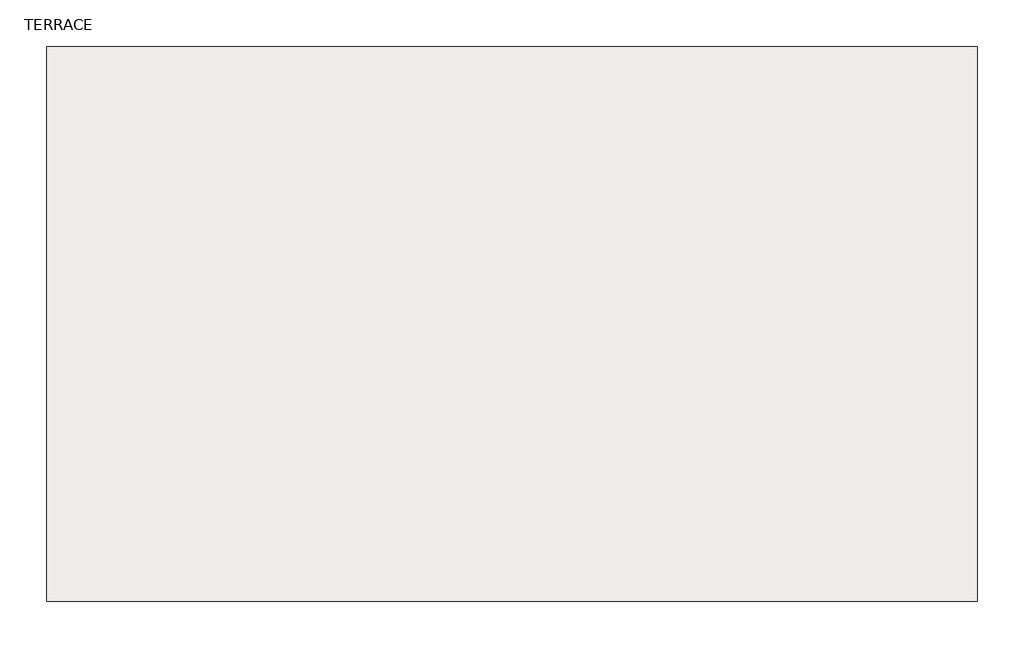
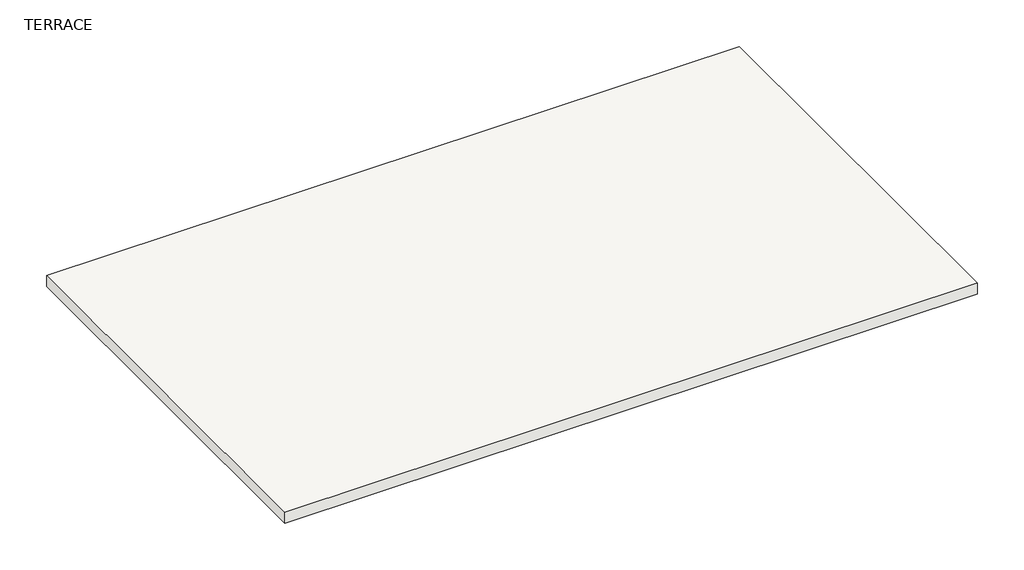
# One storey: 1 slab.
"""IFC4 building model written with IfcOpenShell, lengths in millimetres."""

from ifc_helpers import new_model, si_unit, frame, origin, place, context, project, spatial, polyline, outline, extrude, element, save

model = new_model("IFC4")

# Units and contexts
model_context = context("Model", 3, world=origin())
ifc_project = project(units=[si_unit("LENGTHUNIT", "METRE", prefix="MILLI")], contexts=[model_context])

# Site, building, storey
site = spatial("IfcSite", under=ifc_project)
building = spatial("IfcBuilding", under=site)
storey = spatial("IfcBuildingStorey", under=building, Name="TERRACE", Elevation=12801.6)

# Slab
placement = place(None, origin())
element("IfcSlab", 1, ObjectType="6\" SLAB", at=placement, inside=storey, context=model_context, shape_type="SweptSolid", body=[
    extrude(outline(polyline([(56.4408773, 5407.3642852), (9213.1408773, 5407.3642852), (9213.1408773, -53.6357148), (56.4408773, -53.6357148), (56.4408773, 5407.3642852)])), frame((0.0, 0.0, 12700.0), z_axis=(0.0, 0.0, 1.0), x_axis=(1.0, 0.0, 0.0)), (0.0, 0.0, 1.0), 152.4),
])

save(model, "model.ifc")

# Revit data of these elements
# Type "6\" SLAB"
#   Assembly Code = "B1010"
#   Function = 0
#   Layers, outside or top first: 0' - 6" "Concrete, Lightweight" (function 1)
# Element 1 (IfcSlab, "6\" SLAB")
#   built-in parameter 1001955 = 3.14159 (stored number, unit not read)
#   Height Offset From Level = 0' - 2"
#   Phase Created = New Construction
#   Materials on its faces: "Concrete, Lightweight"
# Materials
#   "Concrete, Lightweight": class "Concrete", colour RGB 142 141 140, transparency 0, Description = "Lightweight concrete", Cost = 0
